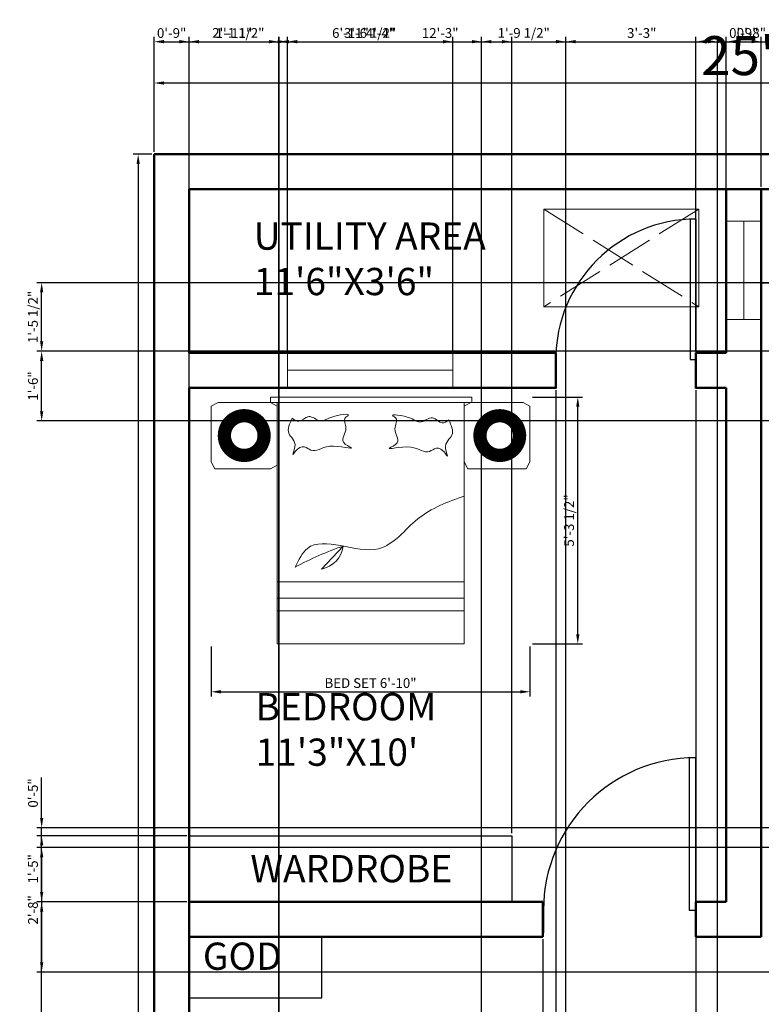
# Model space of a CAD drawing. Units: inches. Extents: x 1854 to 2268, y 1958 to 2535.
# Tile 3 of 4: x 1854 to 2044, y 2283 to 2535. Entities that reach past the tile are written whole.
import ezdxf

# ---------------------------------------------------------------- set-up
doc = ezdxf.new("R2010")
doc.units = ezdxf.units.IN
doc.linetypes.add('ACAD_ISO02W100', pattern=[15, 12, -3])
for name, color, linetype, lineweight in [('A-ANNO-DIMS', 2, 'Continuous', 18), ('A-ANNO-TEXT', 7, 'Continuous', 25), ('A-AREA-IDEN', 7, 'Continuous', 25), ('A-DOOR', 3, 'Continuous', 25), ('A-EQPM', 9, 'Continuous', 18), ('A-EQPM-OVHD', 9, 'ACAD_ISO02W100', 13), ('A-FLOR-CASE', 30, 'Continuous', 25), ('A-FURN', 8, 'Continuous', 18), ('A-GLAZ', 4, 'Continuous', 18), ('A-WALL', 7, 'Continuous', 50)]:
    doc.layers.add(name, color=color, linetype=linetype, lineweight=lineweight)
doc.styles.get("Standard").update_dxf_attribs({"font": 'arial.ttf'})
doc.dimstyles.new('ISO-25', dxfattribs={"dimtxt": 2.5, "dimasz": 2.5, "dimexe": 1.25, "dimexo": 0.625, "dimtad": 1, "dimdec": 0, "dimlunit": 3, "dimtxsty": 'Standard', "dimcen": 2.5, "dimadec": 0, "dimazin": 0, "dimtfac": 1, "dimtdec": 0, "dimtmove": 0, "dimatfit": 3, "dimfxl": 1, "dimarcsym": 0})

# ---------------------------------------------------------------- blocks, each defined once
blk = doc.blocks.new('*U12')
for p, q in [((0, 0), (0, -6)), ((-40, 0), (-40, -6))]:
    blk.add_line(p, q)
blk.add_lwpolyline([(0, 0), (0, 40), (-1.75, 40), (-1.75, 0)], close=True)
blk.add_arc((0, 0), 40, 90, 180)
blk = doc.blocks.new('*D16')
at = {"layer": 'A-ANNO-DIMS', "color": 0, "lineweight": -2, "transparency": 16777216}
for p, q in [((1888.43, 2501.46), (1888.43, 2520.38)), ((1890.93, 2519.13), (2185.93, 2519.13)), ((2188.43, 2501.46), (2188.43, 2520.38))]:
    blk.add_line(p, q, dxfattribs=at)
at = {"layer": 'A-ANNO-DIMS', "color": 0, "transparency": 16777216}
for points in [[(1890.93, 2519.54), (1890.93, 2518.71), (1888.43, 2519.13)], [(2185.93, 2519.54), (2185.93, 2518.71), (2188.43, 2519.13)]]:
    blk.add_solid(points, dxfattribs=at)
at = {"layer": 'Defpoints', "color": 0, "transparency": 16777216}
for p in [(2188.43, 2519.13), (1888.43, 2500.84), (2188.43, 2500.84)]:
    blk.add_point(p, dxfattribs=at)
at = {"layer": 'A-ANNO-DIMS', "color": 0, "transparency": 16777216, "insert": (2038.43, 2524.86), "char_height": 10, "attachment_point": 5}
blk.add_mtext("25'", dxfattribs=at)
blk = doc.blocks.new('*D17')
at = {"layer": 'A-ANNO-DIMS', "color": 0, "lineweight": -2, "transparency": 16777216}
for p, q in [((1887.81, 2500.84), (1883.08, 2500.84)), ((1884.33, 2498.34), (1884.33, 2023.34)), ((1887.81, 2020.84), (1883.08, 2020.84))]:
    blk.add_line(p, q, dxfattribs=at)
at = {"layer": 'A-ANNO-DIMS', "color": 0, "transparency": 16777216}
for points in [[(1883.91, 2498.34), (1884.74, 2498.34), (1884.33, 2500.84)], [(1883.91, 2023.34), (1884.74, 2023.34), (1884.33, 2020.84)]]:
    blk.add_solid(points, dxfattribs=at)
at = {"layer": 'Defpoints', "color": 0, "transparency": 16777216}
for p in [(1888.43, 2500.84), (1884.33, 2020.84), (1888.43, 2020.84)]:
    blk.add_point(p, dxfattribs=at)
at = {"layer": 'A-ANNO-DIMS', "color": 0, "transparency": 16777216, "insert": (1878.6, 2260.84), "char_height": 10, "attachment_point": 5, "rotation": 90}
blk.add_mtext("40'", dxfattribs=at)
blk = doc.blocks.new('BED-DOUBLE-48-WITH-NIGHTSTANDS')
for p, q in [((66.94, 63.4), (15.26, 63.4)), ((15.26, 63.4), (15.26, 62.01)), ((66.94, 62.01), (66.94, 63.4)), ((15.24, 62.01), (66.94, 62.01)), ((66.76, 62.01), (65, 61.07)), ((65, 46.77), (65, 61.07)), ((66.76, 62.01), (80.15, 62.01)), ((80.15, 62.01), (81.91, 61.07)), ((81.91, 61.07), (81.91, 46.77)), ((65, 46.77), (65.94, 45.01)), ((81.91, 46.77), (80.97, 45.01)), ((80.97, 45.01), (65.94, 45.01)), ((65, 33.11), (65, 0.01)), ((33.9, 25.12), (28.32, 19.22)), ((17, 15.97), (65, 15.97)), ((17, 11.74), (65, 11.74)), ((17, 8.47), (65, 8.47)), ((30.83, 0.01), (33.39, 0))]:
    blk.add_line(p, q)
for points in [[(15.24, 62.01), (1.76, 62.01), (0, 61.07), (0, 46.77), (0.94, 45.01), (15.24, 45.01), (17, 45.95), (17, 61.07)], [(17, 62.01), (65, 62.01), (65, 0.01), (17, 0.01)]]:
    blk.add_lwpolyline(points, close=True)
at = {"const_width": 3.4}
for points in [[(3.4, 53.51, 1), (13.6, 53.51, 1)], [(69.06, 53.51, 1), (79.25, 53.51, 1)]]:
    blk.add_lwpolyline(points, format="xyb", close=True, dxfattribs=at)
for centre, radius, start, end in [((59.98, -51.08), 80.54, 108.8924, 118.4699), ((27.17, 25.91), 6.78, 279.7804, 353.3519)]:
    blk.add_arc(centre, radius, start, end)
for points, knots in [([(20.85, 57.96), (21.4, 57.55), (22.81, 56.52), (25.07, 59.43), (28.07, 56.49), (30.47, 58.63), (36.69, 59.38), (33.63, 57.81), (35.62, 55), (32.56, 51.97), (38.38, 49.37), (29.56, 52.01), (26.59, 48.71), (23.73, 51.16), (22.03, 50.08), (20.5, 47.89), (22.53, 51.91), (18.89, 53.83), (20.19, 56.57), (20.85, 57.96)], [0, 0, 0, 0, 1.83091, 4.653214, 7.743318, 10.66504, 15.119925, 15.953636, 18.69724, 22.356007, 24.774329, 30.270914, 35.21341, 37.060797, 39.714351, 40.728626, 42.795822, 46.625816, 50.594847, 50.594847, 50.594847, 50.594847]), ([(61.06, 57.53), (60.49, 57.13), (59.07, 56.13), (56.87, 59.08), (53.81, 56.21), (51.45, 58.4), (45.25, 59.29), (48.28, 57.65), (46.23, 54.88), (49.23, 51.79), (43.35, 49.32), (52.22, 51.77), (55.12, 48.4), (58.03, 50.79), (59.71, 49.68), (61.2, 47.45), (59.25, 51.51), (62.92, 53.35), (61.69, 56.12), (61.06, 57.53)], [0, 0, 0, 0, 1.83091, 4.653214, 7.743318, 10.66504, 15.119925, 15.953636, 18.69724, 22.356007, 24.774329, 30.270914, 35.21341, 37.060797, 39.714351, 40.728626, 42.795822, 46.625816, 50.594847, 50.594847, 50.594847, 50.594847]), ([(65, 37.97), (60.8, 36.46), (52.61, 33.52), (43.01, 19.71), (26.29, 29.43), (22.5, 21.6), (21.59, 19.72)], [0, 0, 0, 0, 13.291621, 25.945947, 44.21489, 49.956985, 49.956985, 49.956985, 49.956985])]:
    blk.add_open_spline(points, degree=3, knots=knots)
blk = doc.blocks.new('*D25')
at = {"layer": 'A-ANNO-DIMS', "color": 0, "lineweight": -2, "transparency": 16777216}
for p, q in [((1903.08, 2374.44), (1903.08, 2361.53)), ((1984.99, 2374.44), (1984.99, 2361.53)), ((1905.58, 2362.78), (1982.49, 2362.78))]:
    blk.add_line(p, q, dxfattribs=at)
at = {"layer": 'A-ANNO-DIMS', "color": 0, "transparency": 16777216}
for points in [[(1905.58, 2363.2), (1905.58, 2362.36), (1903.08, 2362.78)], [(1982.49, 2363.2), (1982.49, 2362.36), (1984.99, 2362.78)]]:
    blk.add_solid(points, dxfattribs=at)
at = {"layer": 'Defpoints', "color": 0, "transparency": 16777216}
for p in [(1903.08, 2375.07), (1984.99, 2375.07), (1984.99, 2362.78)]:
    blk.add_point(p, dxfattribs=at)
at = {"layer": 'A-ANNO-DIMS', "color": 0, "transparency": 16777216, "insert": (1944.03, 2364.7), "char_height": 2.5, "attachment_point": 5}
blk.add_mtext('BED SET 6\'-10"', dxfattribs=at)
blk = doc.blocks.new('*D26')
at = {"layer": 'A-ANNO-DIMS', "color": 0, "lineweight": -2, "transparency": 16777216}
for p, q in [((1985.61, 2438.47), (1998.53, 2438.47)), ((1997.28, 2377.57), (1997.28, 2435.97)), ((1985.61, 2375.07), (1998.53, 2375.07))]:
    blk.add_line(p, q, dxfattribs=at)
at = {"layer": 'A-ANNO-DIMS', "color": 0, "transparency": 16777216}
for points in [[(1996.86, 2435.97), (1997.69, 2435.97), (1997.28, 2438.47)], [(1996.86, 2377.57), (1997.69, 2377.57), (1997.28, 2375.07)]]:
    blk.add_solid(points, dxfattribs=at)
at = {"layer": 'Defpoints', "color": 0, "transparency": 16777216}
for p in [(1984.99, 2438.47), (1997.28, 2438.47), (1984.99, 2375.07)]:
    blk.add_point(p, dxfattribs=at)
at = {"layer": 'A-ANNO-DIMS', "color": 0, "transparency": 16777216, "insert": (1995.36, 2406.77), "char_height": 2.5, "attachment_point": 5, "rotation": 90}
blk.add_mtext('5\'-3 1/2"', dxfattribs=at)
blk = doc.blocks.new('*D31')
at = {"layer": 'A-ANNO-DIMS', "color": 0, "lineweight": -2, "transparency": 16777216}
for p, q in [((1888.43, 2501.46), (1888.43, 2530.99)), ((1890.93, 2529.74), (1894.93, 2529.74)), ((1897.43, 2492.46), (1897.43, 2530.99))]:
    blk.add_line(p, q, dxfattribs=at)
at = {"layer": 'A-ANNO-DIMS', "color": 0, "transparency": 16777216}
for points in [[(1890.93, 2530.16), (1890.93, 2529.32), (1888.43, 2529.74)], [(1894.93, 2530.16), (1894.93, 2529.32), (1897.43, 2529.74)]]:
    blk.add_solid(points, dxfattribs=at)
at = {"layer": 'Defpoints', "color": 0, "transparency": 16777216}
for p in [(1897.43, 2529.74), (1888.43, 2500.84), (1897.43, 2491.84)]:
    blk.add_point(p, dxfattribs=at)
at = {"layer": 'A-ANNO-DIMS', "color": 0, "transparency": 16777216, "insert": (1892.93, 2531.64), "char_height": 2.5, "attachment_point": 5}
blk.add_mtext('0\'-9"', dxfattribs=at)
blk = doc.blocks.new('*D32')
at = {"layer": 'A-ANNO-DIMS', "color": 0, "lineweight": -2, "transparency": 16777216}
for p, q in [((2035.43, 2492.46), (2035.43, 2530.99)), ((2037.93, 2529.74), (2041.93, 2529.74)), ((2044.43, 2492.46), (2044.43, 2530.99))]:
    blk.add_line(p, q, dxfattribs=at)
at = {"layer": 'A-ANNO-DIMS', "color": 0, "transparency": 16777216}
for points in [[(2037.93, 2530.16), (2037.93, 2529.32), (2035.43, 2529.74)], [(2041.93, 2530.16), (2041.93, 2529.32), (2044.43, 2529.74)]]:
    blk.add_solid(points, dxfattribs=at)
at = {"layer": 'Defpoints', "color": 0, "transparency": 16777216}
for p in [(2044.43, 2529.74), (2035.43, 2491.84), (2044.43, 2491.84)]:
    blk.add_point(p, dxfattribs=at)
at = {"layer": 'A-ANNO-DIMS', "color": 0, "transparency": 16777216, "insert": (2039.93, 2531.64), "char_height": 2.5, "attachment_point": 5}
blk.add_mtext('0\'-9"', dxfattribs=at)
blk = doc.blocks.new('*D33')
at = {"layer": 'A-ANNO-DIMS', "color": 0, "lineweight": -2, "transparency": 16777216}
for p, q in [((1991.6, 2440.21), (1991.6, 1966.69)), ((2027.6, 2440.21), (2027.6, 1966.69)), ((1994.1, 1967.94), (2025.1, 1967.94))]:
    blk.add_line(p, q, dxfattribs=at)
at = {"layer": 'A-ANNO-DIMS', "color": 0, "transparency": 16777216}
for points in [[(1994.1, 1968.36), (1994.1, 1967.52), (1991.6, 1967.94)], [(2025.1, 1968.36), (2025.1, 1967.52), (2027.6, 1967.94)]]:
    blk.add_solid(points, dxfattribs=at)
at = {"layer": 'Defpoints', "color": 0, "transparency": 16777216}
for p in [(1991.6, 2440.84), (2027.6, 2440.84), (2027.6, 1967.94)]:
    blk.add_point(p, dxfattribs=at)
at = {"layer": 'A-ANNO-DIMS', "color": 0, "transparency": 16777216, "insert": (2009.6, 1969.84), "char_height": 2.5, "attachment_point": 5}
blk.add_mtext('3\'-0"', dxfattribs=at)
blk = doc.blocks.new('*D34')
at = {"layer": 'A-ANNO-DIMS', "color": 0, "lineweight": -2, "transparency": 16777216}
for p, q in [((1922.69, 2450.46), (1922.69, 2530.99)), ((1925.19, 2529.74), (1962.64, 2529.74)), ((1965.14, 2450.46), (1965.14, 2530.99))]:
    blk.add_line(p, q, dxfattribs=at)
at = {"layer": 'A-ANNO-DIMS', "color": 0, "transparency": 16777216}
for points in [[(1925.19, 2530.16), (1925.19, 2529.32), (1922.69, 2529.74)], [(1962.64, 2530.16), (1962.64, 2529.32), (1965.14, 2529.74)]]:
    blk.add_solid(points, dxfattribs=at)
at = {"layer": 'Defpoints', "color": 0, "transparency": 16777216}
for p in [(1965.14, 2529.74), (1922.69, 2449.84), (1965.14, 2449.84)]:
    blk.add_point(p, dxfattribs=at)
at = {"layer": 'A-ANNO-DIMS', "color": 0, "transparency": 16777216, "insert": (1943.91, 2531.66), "char_height": 2.5, "attachment_point": 5}
blk.add_mtext('3\'-6 1/2"', dxfattribs=at)
blk = doc.blocks.new('*D35')
at = {"layer": 'A-ANNO-DIMS', "color": 0, "lineweight": -2, "transparency": 16777216}
for p, q in [((1988.27, 2299.21), (1988.27, 1966.69)), ((2027.59, 2299.21), (2027.59, 1966.69)), ((1990.77, 1967.94), (2025.09, 1967.94))]:
    blk.add_line(p, q, dxfattribs=at)
at = {"layer": 'A-ANNO-DIMS', "color": 0, "transparency": 16777216}
for points in [[(1990.77, 1968.36), (1990.77, 1967.52), (1988.27, 1967.94)], [(2025.09, 1968.36), (2025.09, 1967.52), (2027.59, 1967.94)]]:
    blk.add_solid(points, dxfattribs=at)
at = {"layer": 'Defpoints', "color": 0, "transparency": 16777216}
for p in [(1988.27, 2299.84), (2027.59, 2299.84), (2027.59, 1967.94)]:
    blk.add_point(p, dxfattribs=at)
at = {"layer": 'A-ANNO-DIMS', "color": 0, "transparency": 16777216, "insert": (2007.93, 1969.86), "char_height": 2.5, "attachment_point": 5}
blk.add_mtext('3\'-3 1/2"', dxfattribs=at)
blk = doc.blocks.new('*D37')
at = {"layer": 'A-ANNO-DIMS', "color": 0, "lineweight": -2, "transparency": 16777216}
for p, q in [((2113.81, 2322.77), (1858.28, 2322.77)), ((1859.53, 2320.27), (1859.53, 2293.27)), ((2113.81, 2290.77), (1858.28, 2290.77))]:
    blk.add_line(p, q, dxfattribs=at)
at = {"layer": 'A-ANNO-DIMS', "color": 0, "transparency": 16777216}
for points in [[(1859.12, 2320.27), (1859.95, 2320.27), (1859.53, 2322.77)], [(1859.12, 2293.27), (1859.95, 2293.27), (1859.53, 2290.77)]]:
    blk.add_solid(points, dxfattribs=at)
at = {"layer": 'Defpoints', "color": 0, "transparency": 16777216}
for p in [(2114.43, 2322.77), (1859.53, 2290.77), (2114.43, 2290.77)]:
    blk.add_point(p, dxfattribs=at)
at = {"layer": 'A-ANNO-DIMS', "color": 0, "transparency": 16777216, "insert": (1857.63, 2306.77), "char_height": 2.5, "attachment_point": 5, "rotation": 90}
blk.add_mtext('2\'-8"', dxfattribs=at)
blk = doc.blocks.new('*D39')
at = {"layer": 'A-ANNO-DIMS', "color": 0, "lineweight": -2, "transparency": 16777216}
for p, q in [((1920.58, 2131.39), (1920.58, 2530.99)), ((1923.08, 2529.74), (1970.08, 2529.74)), ((1972.58, 2131.39), (1972.58, 2530.99))]:
    blk.add_line(p, q, dxfattribs=at)
at = {"layer": 'A-ANNO-DIMS', "color": 0, "transparency": 16777216}
for points in [[(1923.08, 2530.16), (1923.08, 2529.32), (1920.58, 2529.74)], [(1970.08, 2530.16), (1970.08, 2529.32), (1972.58, 2529.74)]]:
    blk.add_solid(points, dxfattribs=at)
at = {"layer": 'Defpoints', "color": 0, "transparency": 16777216}
for p in [(1972.58, 2529.74), (1920.58, 2130.77), (1972.58, 2130.77)]:
    blk.add_point(p, dxfattribs=at)
at = {"layer": 'A-ANNO-DIMS', "color": 0, "transparency": 16777216, "insert": (1946.58, 2531.61), "char_height": 2.5, "attachment_point": 5}
blk.add_mtext('4\'-4"', dxfattribs=at)
blk = doc.blocks.new('*D40')
at = {"layer": 'A-ANNO-DIMS', "color": 0, "lineweight": -2, "transparency": 16777216}
for p, q in [((1897.43, 2135.46), (1897.43, 2530.99)), ((1899.93, 2529.74), (1917.95, 2529.74)), ((1920.45, 2135.35), (1920.45, 2530.99))]:
    blk.add_line(p, q, dxfattribs=at)
at = {"layer": 'A-ANNO-DIMS', "color": 0, "transparency": 16777216}
for points in [[(1899.93, 2530.16), (1899.93, 2529.32), (1897.43, 2529.74)], [(1917.95, 2530.16), (1917.95, 2529.32), (1920.45, 2529.74)]]:
    blk.add_solid(points, dxfattribs=at)
at = {"layer": 'Defpoints', "color": 0, "transparency": 16777216}
for p in [(1920.45, 2529.74), (1897.43, 2134.84), (1920.45, 2134.72)]:
    blk.add_point(p, dxfattribs=at)
at = {"layer": 'A-ANNO-DIMS', "color": 0, "transparency": 16777216, "insert": (1908.94, 2531.62), "char_height": 2.5, "attachment_point": 5}
blk.add_mtext('1\'-11"', dxfattribs=at)
blk = doc.blocks.new('*D41')
at = {"layer": 'A-ANNO-DIMS', "color": 0, "lineweight": -2, "transparency": 16777216}
for p, q in [((1972.58, 2135.49), (1972.58, 2530.99)), ((1975.08, 2529.74), (1991.71, 2529.74)), ((1994.21, 2135.46), (1994.21, 2530.99))]:
    blk.add_line(p, q, dxfattribs=at)
at = {"layer": 'A-ANNO-DIMS', "color": 0, "transparency": 16777216}
for points in [[(1975.08, 2530.16), (1975.08, 2529.32), (1972.58, 2529.74)], [(1991.71, 2530.16), (1991.71, 2529.32), (1994.21, 2529.74)]]:
    blk.add_solid(points, dxfattribs=at)
at = {"layer": 'Defpoints', "color": 0, "transparency": 16777216}
for p in [(1994.21, 2529.74), (1972.58, 2134.87), (1994.21, 2134.84)]:
    blk.add_point(p, dxfattribs=at)
at = {"layer": 'A-ANNO-DIMS', "color": 0, "transparency": 16777216, "insert": (1983.39, 2531.66), "char_height": 2.5, "attachment_point": 5}
blk.add_mtext('1\'-9 1/2"', dxfattribs=at)
blk = doc.blocks.new('*D42')
at = {"layer": 'A-ANNO-DIMS', "color": 0, "lineweight": -2, "transparency": 16777216}
for p, q in [((1994.21, 2135.46), (1994.21, 2530.99)), ((1996.71, 2529.74), (2030.71, 2529.74)), ((2033.21, 2135.46), (2033.21, 2530.99))]:
    blk.add_line(p, q, dxfattribs=at)
at = {"layer": 'A-ANNO-DIMS', "color": 0, "transparency": 16777216}
for points in [[(1996.71, 2530.16), (1996.71, 2529.32), (1994.21, 2529.74)], [(2030.71, 2530.16), (2030.71, 2529.32), (2033.21, 2529.74)]]:
    blk.add_solid(points, dxfattribs=at)
at = {"layer": 'Defpoints', "color": 0, "transparency": 16777216}
for p in [(2033.21, 2529.74), (1994.21, 2134.84), (2033.21, 2134.84)]:
    blk.add_point(p, dxfattribs=at)
at = {"layer": 'A-ANNO-DIMS', "color": 0, "transparency": 16777216, "insert": (2013.71, 2531.64), "char_height": 2.5, "attachment_point": 5}
blk.add_mtext('3\'-3"', dxfattribs=at)
blk = doc.blocks.new('*D50')
at = {"layer": 'A-ANNO-DIMS', "color": 0, "lineweight": -2, "transparency": 16777216}
for p, q in [((1897.43, 2450.46), (1897.43, 2530.99)), ((1899.93, 2529.74), (1920.19, 2529.74)), ((1922.69, 2450.46), (1922.69, 2530.99))]:
    blk.add_line(p, q, dxfattribs=at)
at = {"layer": 'A-ANNO-DIMS', "color": 0, "transparency": 16777216}
for points in [[(1899.93, 2530.16), (1899.93, 2529.32), (1897.43, 2529.74)], [(1920.19, 2530.16), (1920.19, 2529.32), (1922.69, 2529.74)]]:
    blk.add_solid(points, dxfattribs=at)
at = {"layer": 'Defpoints', "color": 0, "transparency": 16777216}
for p in [(1922.69, 2529.74), (1897.43, 2449.84), (1922.69, 2449.84)]:
    blk.add_point(p, dxfattribs=at)
at = {"layer": 'A-ANNO-DIMS', "color": 0, "transparency": 16777216, "insert": (1910.06, 2531.66), "char_height": 2.5, "attachment_point": 5}
blk.add_mtext('2\'-1 1/2"', dxfattribs=at)
blk = doc.blocks.new('*D51')
at = {"layer": 'A-ANNO-DIMS', "color": 0, "lineweight": -2, "transparency": 16777216}
for p, q in [((2027.6, 2450.46), (2027.6, 2530.99)), ((2030.1, 2529.74), (2032.93, 2529.74)), ((2035.43, 2450.46), (2035.43, 2530.99)), ((2035.43, 2529.74), (2045.83, 2529.74))]:
    blk.add_line(p, q, dxfattribs=at)
at = {"layer": 'A-ANNO-DIMS', "color": 0, "transparency": 16777216}
for points in [[(2030.1, 2530.16), (2030.1, 2529.32), (2027.6, 2529.74)], [(2032.93, 2530.16), (2032.93, 2529.32), (2035.43, 2529.74)]]:
    blk.add_solid(points, dxfattribs=at)
at = {"layer": 'Defpoints', "color": 0, "transparency": 16777216}
for p in [(2035.43, 2529.74), (2027.6, 2449.84), (2035.43, 2449.84)]:
    blk.add_point(p, dxfattribs=at)
at = {"layer": 'A-ANNO-DIMS', "color": 0, "transparency": 16777216, "insert": (2041.88, 2531.64), "char_height": 2.5, "attachment_point": 5}
blk.add_mtext('0\'-8"', dxfattribs=at)
blk = doc.blocks.new('*D54')
at = {"layer": 'A-ANNO-DIMS', "color": 0, "lineweight": -2, "transparency": 16777216}
for p, q in [((1888.43, 2501.46), (1888.43, 2530.99)), ((1890.93, 2529.74), (2032.93, 2529.74)), ((2035.43, 2492.46), (2035.43, 2530.99))]:
    blk.add_line(p, q, dxfattribs=at)
at = {"layer": 'A-ANNO-DIMS', "color": 0, "transparency": 16777216}
for points in [[(1890.93, 2530.16), (1890.93, 2529.32), (1888.43, 2529.74)], [(2032.93, 2530.16), (2032.93, 2529.32), (2035.43, 2529.74)]]:
    blk.add_solid(points, dxfattribs=at)
at = {"layer": 'Defpoints', "color": 0, "transparency": 16777216}
for p in [(2035.43, 2529.74), (1888.43, 2500.84), (2035.43, 2491.84)]:
    blk.add_point(p, dxfattribs=at)
at = {"layer": 'A-ANNO-DIMS', "color": 0, "transparency": 16777216, "insert": (1961.93, 2531.64), "char_height": 2.5, "attachment_point": 5}
blk.add_mtext('12\'-3"', dxfattribs=at)
blk = doc.blocks.new('*D68')
at = {"layer": 'A-ANNO-DIMS', "color": 0, "lineweight": -2, "transparency": 16777216}
for p, q in [((1896.81, 2308.84), (1858.28, 2308.84)), ((1859.53, 2023.34), (1859.53, 2306.34)), ((1887.81, 2020.84), (1858.28, 2020.84))]:
    blk.add_line(p, q, dxfattribs=at)
at = {"layer": 'A-ANNO-DIMS', "color": 0, "transparency": 16777216}
for points in [[(1859.12, 2306.34), (1859.95, 2306.34), (1859.53, 2308.84)], [(1859.12, 2023.34), (1859.95, 2023.34), (1859.53, 2020.84)]]:
    blk.add_solid(points, dxfattribs=at)
at = {"layer": 'Defpoints', "color": 0, "transparency": 16777216}
for p in [(1859.53, 2308.84), (1897.43, 2308.84), (1888.43, 2020.84)]:
    blk.add_point(p, dxfattribs=at)
at = {"layer": 'A-ANNO-DIMS', "color": 0, "transparency": 16777216, "insert": (1857.63, 2164.84), "char_height": 2.5, "attachment_point": 5, "rotation": 90}
blk.add_mtext('24\'-0"', dxfattribs=at)
blk = doc.blocks.new('*D70')
at = {"layer": 'A-ANNO-DIMS', "color": 0, "lineweight": -2, "transparency": 16777216}
for p, q in [((1859.53, 2330.34), (1859.53, 2340.74)), ((2113.81, 2327.84), (1858.28, 2327.84)), ((1859.53, 2322.77), (1859.53, 2327.84)), ((2113.81, 2322.77), (1858.28, 2322.77)), ((1859.53, 2320.27), (1859.53, 2317.77))]:
    blk.add_line(p, q, dxfattribs=at)
at = {"layer": 'A-ANNO-DIMS', "color": 0, "transparency": 16777216}
for points in [[(1859.12, 2330.34), (1859.95, 2330.34), (1859.53, 2327.84)], [(1859.12, 2320.27), (1859.95, 2320.27), (1859.53, 2322.77)]]:
    blk.add_solid(points, dxfattribs=at)
at = {"layer": 'Defpoints', "color": 0, "transparency": 16777216}
for p in [(1859.53, 2327.84), (2114.43, 2327.84), (2114.43, 2322.77)]:
    blk.add_point(p, dxfattribs=at)
at = {"layer": 'A-ANNO-DIMS', "color": 0, "transparency": 16777216, "insert": (1857.63, 2336.79), "char_height": 2.5, "attachment_point": 5, "rotation": 90}
blk.add_mtext('0\'-5"', dxfattribs=at)
blk = doc.blocks.new('*D73')
at = {"layer": 'A-ANNO-DIMS', "color": 0, "lineweight": -2, "transparency": 16777216}
for p, q in [((2159.76, 2450.27), (1858.28, 2450.27)), ((1859.53, 2434.83), (1859.53, 2447.77)), ((2159.76, 2432.33), (1858.28, 2432.33))]:
    blk.add_line(p, q, dxfattribs=at)
at = {"layer": 'A-ANNO-DIMS', "color": 0, "transparency": 16777216}
for points in [[(1859.12, 2447.77), (1859.95, 2447.77), (1859.53, 2450.27)], [(1859.12, 2434.83), (1859.95, 2434.83), (1859.53, 2432.33)]]:
    blk.add_solid(points, dxfattribs=at)
at = {"layer": 'Defpoints', "color": 0, "transparency": 16777216}
for p in [(1859.53, 2450.27), (2160.38, 2450.27), (2160.38, 2432.33)]:
    blk.add_point(p, dxfattribs=at)
at = {"layer": 'A-ANNO-DIMS', "color": 0, "transparency": 16777216, "insert": (1857.63, 2441.3), "char_height": 2.5, "attachment_point": 5, "rotation": 90}
blk.add_mtext('1\'-6"', dxfattribs=at)
blk = doc.blocks.new('*D74')
at = {"layer": 'A-ANNO-DIMS', "color": 0, "lineweight": -2, "transparency": 16777216}
for p, q in [((2154.81, 2467.84), (1858.28, 2467.84)), ((1859.53, 2452.77), (1859.53, 2465.34)), ((2159.76, 2450.27), (1858.28, 2450.27))]:
    blk.add_line(p, q, dxfattribs=at)
at = {"layer": 'A-ANNO-DIMS', "color": 0, "transparency": 16777216}
for points in [[(1859.12, 2465.34), (1859.95, 2465.34), (1859.53, 2467.84)], [(1859.12, 2452.77), (1859.95, 2452.77), (1859.53, 2450.27)]]:
    blk.add_solid(points, dxfattribs=at)
at = {"layer": 'Defpoints', "color": 0, "transparency": 16777216}
for p in [(1859.53, 2467.84), (2155.43, 2467.84), (2160.38, 2450.27)]:
    blk.add_point(p, dxfattribs=at)
at = {"layer": 'A-ANNO-DIMS', "color": 0, "transparency": 16777216, "insert": (1857.61, 2459.05), "char_height": 2.5, "attachment_point": 5, "rotation": 90}
blk.add_mtext('1\'-5 1/2"', dxfattribs=at)
blk = doc.blocks.new('*D75')
at = {"layer": 'A-ANNO-DIMS', "color": 0, "lineweight": -2, "transparency": 16777216}
for p, q in [((1897.43, 2326.43), (1897.43, 2530.99)), ((1899.93, 2529.74), (1977.8, 2529.74)), ((1980.3, 2326.43), (1980.3, 2530.99))]:
    blk.add_line(p, q, dxfattribs=at)
at = {"layer": 'A-ANNO-DIMS', "color": 0, "transparency": 16777216}
for points in [[(1899.93, 2530.16), (1899.93, 2529.32), (1897.43, 2529.74)], [(1977.8, 2530.16), (1977.8, 2529.32), (1980.3, 2529.74)]]:
    blk.add_solid(points, dxfattribs=at)
at = {"layer": 'Defpoints', "color": 0, "transparency": 16777216}
for p in [(1980.3, 2529.74), (1897.43, 2325.81), (1980.3, 2325.81)]:
    blk.add_point(p, dxfattribs=at)
at = {"layer": 'A-ANNO-DIMS', "color": 0, "transparency": 16777216, "insert": (1938.87, 2531.64), "char_height": 2.5, "attachment_point": 5}
blk.add_mtext('6\'-11"', dxfattribs=at)
blk = doc.blocks.new('*D76')
at = {"layer": 'A-ANNO-DIMS', "color": 0, "lineweight": -2, "transparency": 16777216}
for p, q in [((1896.81, 2325.81), (1858.28, 2325.81)), ((1859.53, 2311.34), (1859.53, 2323.31)), ((1896.81, 2308.84), (1858.28, 2308.84))]:
    blk.add_line(p, q, dxfattribs=at)
at = {"layer": 'A-ANNO-DIMS', "color": 0, "transparency": 16777216}
for points in [[(1859.12, 2323.31), (1859.95, 2323.31), (1859.53, 2325.81)], [(1859.12, 2311.34), (1859.95, 2311.34), (1859.53, 2308.84)]]:
    blk.add_solid(points, dxfattribs=at)
at = {"layer": 'Defpoints', "color": 0, "transparency": 16777216}
for p in [(1859.53, 2325.81), (1897.43, 2325.81), (1897.43, 2308.84)]:
    blk.add_point(p, dxfattribs=at)
at = {"layer": 'A-ANNO-DIMS', "color": 0, "transparency": 16777216, "insert": (1857.63, 2317.32), "char_height": 2.5, "attachment_point": 5, "rotation": 90}
blk.add_mtext('1\'-5"', dxfattribs=at)

msp = doc.modelspace()

# ---------------------------------------------------------------- linework, layer by layer
at = {"layer": 'A-EQPM'}
for p, q in [((1988.54, 2486.75), (2028.36, 2486.75)), ((1988.54, 2461.64), (1988.54, 2486.75)), ((2028.36, 2486.75), (2028.36, 2461.64)), ((2028.36, 2461.64), (1988.54, 2461.64))]:
    msp.add_line(p, q, dxfattribs=at)
at = {"layer": 'A-EQPM-OVHD'}
for p, q in [((1988.54, 2486.75), (2028.36, 2461.64)), ((2028.36, 2486.75), (1988.54, 2461.64))]:
    msp.add_line(p, q, dxfattribs=at)
at = {"layer": 'A-FLOR-CASE'}
for p, q in [((2044.43, 2467.84), (2155.43, 2467.84)), ((1897.43, 2325.81), (1980.3, 2325.81)), ((1980.3, 2325.81), (1980.3, 2308.84)), ((1931.48, 2284.18), (1931.48, 2299.84)), ((1897.43, 2284.18), (1931.48, 2284.18))]:
    msp.add_line(p, q, dxfattribs=at)
at = {"layer": 'A-GLAZ'}
for p, q in [((2035.43, 2483.65), (2044.43, 2483.65)), ((2039.93, 2483.65), (2039.93, 2458.43)), ((2039.93, 2458.43), (2035.43, 2458.43)), ((2035.43, 2458.43), (2044.43, 2458.43)), ((1922.69, 2449.84), (1922.69, 2440.84)), ((1965.14, 2445.34), (1965.14, 2449.84)), ((1965.14, 2449.84), (1965.14, 2440.84)), ((1922.69, 2445.34), (1965.14, 2445.34))]:
    msp.add_line(p, q, dxfattribs=at)
at = {"layer": 'A-WALL'}
for p, q in [((1897.43, 2491.84), (2179.43, 2491.84)), ((1897.43, 2449.84), (1897.43, 2491.84)), ((2035.43, 2449.84), (2035.43, 2491.84)), ((2044.43, 2299.84), (2044.43, 2491.84)), ((1897.43, 2449.84), (1991.6, 2449.84)), ((1991.6, 2449.84), (1991.6, 2440.66)), ((2027.6, 2449.84), (2027.6, 2440.66)), ((2027.6, 2449.84), (2035.43, 2449.84)), ((1897.43, 2029.84), (1897.43, 2440.84)), ((1897.43, 2440.84), (1991.6, 2440.84)), ((1989.59, 2440.9), (1989.59, 2440.84)), ((2027.6, 2440.84), (2035.43, 2440.84)), ((2035.43, 2308.84), (2035.43, 2440.84)), ((1897.43, 2308.84), (1988.27, 2308.84)), ((1988.27, 2308.84), (1988.27, 2299.84)), ((2027.59, 2308.84), (2027.59, 2299.84)), ((2027.59, 2308.84), (2035.43, 2308.84)), ((1897.43, 2299.84), (1988.27, 2299.84)), ((2027.59, 2299.84), (2044.43, 2299.84))]:
    msp.add_line(p, q, dxfattribs=at)
msp.add_lwpolyline([(1888.43, 2500.84), (2188.43, 2500.84), (2188.43, 2020.84), (1888.43, 2020.84)], close=True, dxfattribs=at)

# ---------------------------------------------------------------- block references
at = {"layer": 'A-DOOR'}
for p, xscale, yscale, zscale in [((2027.73, 2448.09), 0.9027437297346877, 0.9027437297346877, 0.9027437297346877), ((2027.6, 2306.73), 0.9781671175203994, 0.9781671175203994, 0.9781671175203994)]:
    msp.add_blockref('*U12', p, dxfattribs=dict(at, xscale=xscale, yscale=yscale, zscale=zscale))
at = {"layer": 'A-FURN'}
msp.add_blockref('BED-DOUBLE-48-WITH-NIGHTSTANDS', (1903.08, 2375.07), dxfattribs=at)

# ---------------------------------------------------------------- texts
at = {"layer": 'A-ANNO-TEXT', "char_height": 7, "attachment_point": 1}
for s, insert in [('WARDROBE', (1913.16, 2320.85)), ('GOD', (1900.96, 2298.37))]:
    msp.add_mtext_dynamic_manual_height_columns(s, width=76.0498, gutter_width=12.5, heights=[0], dxfattribs=dict(at, insert=insert))
at = {"layer": 'A-AREA-IDEN', "char_height": 7, "attachment_point": 1}
for s, insert in [('UTILITY AREA\\P11\'6"X3\'6"', (1914.02, 2483.31)), ('BEDROOM\\P11\'3"X10\'', (1914.49, 2362.44))]:
    msp.add_mtext_dynamic_manual_height_columns(s, width=76.0498, gutter_width=12.5, heights=[0], dxfattribs=dict(at, insert=insert))

# ---------------------------------------------------------------- dimensions: what is measured, and where the dimension line sits
at = {"layer": 'A-ANNO-DIMS'}
for base, p1, p2, override, picture, middle in [((1922.69, 2529.74), (1897.43, 2449.84), (1922.69, 2449.84), {"dimdec": 1, "dimlfac": 1, "dimrnd": 0, "dimzin": 1, "dimdsep": 46, "dimlunit": 4, "dimfrac": 2}, '*D50', (1910.06, 2531.66)), ((1965.1366, 2529.7396), (1922.6914, 2449.8396), (1965.1366, 2449.8396), {"dimdec": 1, "dimlfac": 1, "dimrnd": 0, "dimzin": 1, "dimdsep": 46, "dimlunit": 4, "dimfrac": 2}, '*D34', (1943.914, 2531.6581)), ((1994.21, 2529.74), (1972.58, 2134.87), (1994.21, 2134.84), {"dimdec": 1, "dimlfac": 1, "dimrnd": 0, "dimzin": 1, "dimdsep": 46, "dimlunit": 4, "dimfrac": 2}, '*D41', (1983.39, 2531.66)), ((2035.43, 2529.74), (1888.43, 2500.84), (2035.43, 2491.84), {"dimdec": 1, "dimlfac": 1, "dimrnd": 0, "dimzin": 1, "dimdsep": 46, "dimlunit": 4, "dimfrac": 2}, '*D54', (1961.93, 2531.64)), ((1897.43, 2529.74), (1888.43, 2500.84), (1897.43, 2491.84), {"dimdec": 1, "dimlfac": 1, "dimrnd": 0, "dimzin": 1, "dimdsep": 46, "dimlunit": 4, "dimfrac": 2}, '*D31', (1892.93, 2531.64)), ((2188.43, 2519.13), (1888.43, 2500.84), (2188.43, 2500.84), {"dimtxt": 10, "dimclrd": 0, "dimclre": 0, "dimclrt": 0}, '*D16', (2038.43, 2524.86)), ((1980.3, 2529.74), (1897.43, 2325.81), (1980.3, 2325.81), {"dimdec": 1, "dimlfac": 1, "dimrnd": 0, "dimzin": 1, "dimdsep": 46, "dimlunit": 4, "dimfrac": 2}, '*D75', (1938.87, 2531.64)), ((1920.45, 2529.74), (1897.43, 2134.84), (1920.45, 2134.72), {"dimdec": 1, "dimlfac": 1, "dimrnd": 0, "dimzin": 1, "dimdsep": 46, "dimlunit": 4, "dimfrac": 2}, '*D40', (1908.94, 2531.62)), ((1972.58, 2529.74), (1920.58, 2130.77), (1972.58, 2130.77), {"dimdec": 1, "dimlfac": 1, "dimrnd": 0, "dimzin": 1, "dimdsep": 46, "dimlunit": 4, "dimfrac": 2}, '*D39', (1946.58, 2531.61)), ((2033.21, 2529.74), (1994.21, 2134.84), (2033.21, 2134.84), {"dimdec": 1, "dimlfac": 1, "dimrnd": 0, "dimzin": 1, "dimdsep": 46, "dimlunit": 4, "dimfrac": 2}, '*D42', (2013.71, 2531.64)), ((2035.43, 2529.74), (2027.6, 2449.84), (2035.43, 2449.84), {"dimdec": 1, "dimlfac": 1, "dimrnd": 0, "dimzin": 1, "dimdsep": 46, "dimlunit": 4, "dimfrac": 2}, '*D51', (2041.88, 2531.64)), ((2044.43, 2529.74), (2035.43, 2491.84), (2044.43, 2491.84), {"dimdec": 1, "dimlfac": 1, "dimrnd": 0, "dimzin": 1, "dimdsep": 46, "dimlunit": 4, "dimfrac": 2}, '*D32', (2039.93, 2531.64)), ((2027.6, 1967.94), (1991.6, 2440.84), (2027.6, 2440.84), {"dimdec": 1, "dimlfac": 1, "dimrnd": 0, "dimzin": 1, "dimdsep": 46, "dimlunit": 4, "dimfrac": 2}, '*D33', (2009.6, 1969.84)), ((2027.59, 1967.94), (1988.27, 2299.84), (2027.59, 2299.84), {"dimdec": 1, "dimlfac": 1, "dimrnd": 0, "dimzin": 1, "dimdsep": 46, "dimlunit": 4, "dimfrac": 2}, '*D35', (2007.93, 1969.86))]:
    dim = msp.add_linear_dim(base=base, p1=p1, p2=p2, dimstyle='ISO-25', override=override, dxfattribs=at)
    dim.commit()
    dim.dimension.update_dxf_attribs({"geometry": picture, "text_midpoint": middle})
for base, p1, p2, override, picture, middle in [((1884.33, 2020.84), (1888.43, 2500.84), (1888.43, 2020.84), {"dimtxt": 10, "dimclrd": 0, "dimclre": 0, "dimclrt": 0}, '*D17', (1878.6, 2260.84)), ((1859.53, 2467.84), (2160.38, 2450.27), (2155.43, 2467.84), {"dimdec": 1, "dimlfac": 1, "dimrnd": 0, "dimzin": 1, "dimdsep": 46, "dimlunit": 4, "dimfrac": 2}, '*D74', (1857.61, 2459.05)), ((1859.53, 2450.27), (2160.38, 2432.33), (2160.38, 2450.27), {"dimdec": 1, "dimlfac": 1, "dimrnd": 0, "dimzin": 1, "dimdsep": 46, "dimlunit": 4, "dimfrac": 2}, '*D73', (1857.63, 2441.3)), ((1997.28, 2438.47), (1984.99, 2375.07), (1984.99, 2438.47), {"dimdec": 1, "dimlfac": 1, "dimrnd": 0, "dimzin": 1, "dimdsep": 46, "dimlunit": 4, "dimfrac": 2}, '*D26', (1995.36, 2406.77)), ((1859.53, 2327.84), (2114.43, 2322.77), (2114.43, 2327.84), {"dimdec": 1, "dimlfac": 1, "dimrnd": 0, "dimzin": 1, "dimdsep": 46, "dimlunit": 4, "dimfrac": 2}, '*D70', (1857.63, 2336.79)), ((1859.53, 2325.81), (1897.43, 2308.84), (1897.43, 2325.81), {"dimdec": 1, "dimlfac": 1, "dimrnd": 0, "dimzin": 1, "dimdsep": 46, "dimlunit": 4, "dimfrac": 2}, '*D76', (1857.63, 2317.32)), ((1859.53, 2290.77), (2114.43, 2322.77), (2114.43, 2290.77), {"dimdec": 1, "dimlfac": 1, "dimrnd": 0, "dimzin": 1, "dimdsep": 46, "dimlunit": 4, "dimfrac": 2}, '*D37', (1857.63, 2306.77)), ((1859.53, 2308.84), (1888.43, 2020.84), (1897.43, 2308.84), {"dimdec": 1, "dimlfac": 1, "dimrnd": 0, "dimzin": 1, "dimdsep": 46, "dimlunit": 4, "dimfrac": 2}, '*D68', (1857.63, 2164.84))]:
    dim = msp.add_linear_dim(base=base, p1=p1, p2=p2, angle=90, dimstyle='ISO-25', override=override, dxfattribs=at)
    dim.commit()
    dim.dimension.update_dxf_attribs({"geometry": picture, "text_midpoint": middle})
dim = msp.add_linear_dim(base=(1984.99, 2362.78), p1=(1903.08, 2375.07), p2=(1984.99, 2375.07), text='BED SET <>', dimstyle='ISO-25', override={"dimdec": 1, "dimlfac": 1, "dimrnd": 0, "dimzin": 1, "dimdsep": 46, "dimlunit": 4, "dimfrac": 2}, dxfattribs=at)
dim.commit()
dim.dimension.update_dxf_attribs({"geometry": '*D25', "text_midpoint": (1944.03, 2364.7)})

doc.saveas('drawing.dxf')
